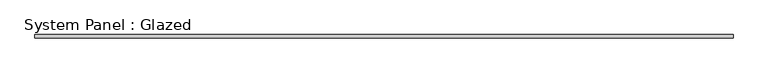
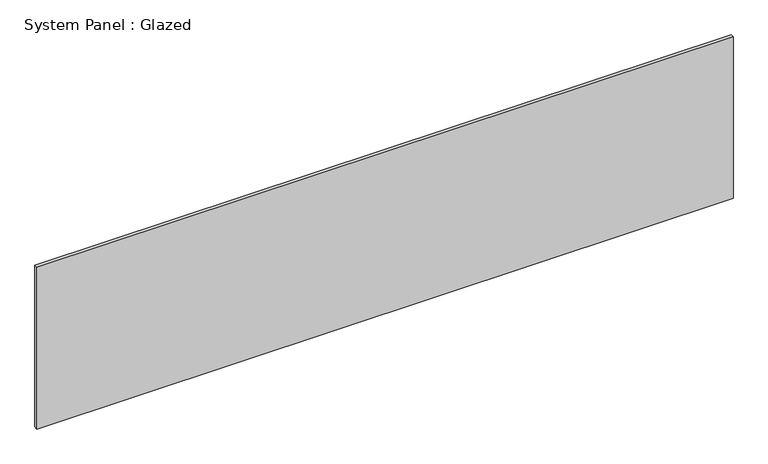
"""IFC4 building model written with IfcOpenShell, lengths in millimetres: plate geometry, System Panel : Glazed."""

from ifc_helpers import new_model, si_unit, origin, origin_with_axes, place, context, project, spatial, polyline, outline, extrude, source, transform, mapped, element, save


def system_panel_glazed_6393fe79(model_context):
    return source(origin(), model_context, "Body", "SweptSolid", [
        extrude(outline(polyline([(2484.742304, 19.05), (-2484.742304, 19.05), (-2484.742304, 44.45), (2484.742304, 44.45), (2484.742304, 19.05)])), origin_with_axes(), (0.0, 0.0, 1.0), 1219.2),
    ])


if __name__ == "__main__":
    model = new_model("IFC4")
    model_context = context("Model", 3, world=origin())
    ifc_project = project(units=[si_unit("LENGTHUNIT", "METRE", prefix="MILLI")], contexts=[model_context])
    site = spatial("IfcSite", under=ifc_project)
    building = spatial("IfcBuilding", under=site)
    placement = place(None, origin())
    system_panel_glazed_shape = system_panel_glazed_6393fe79(model_context)
    element("IfcPlate", 1, ObjectType="System Panel : Glazed", at=placement, inside=building, context=model_context, shape_type="MappedRepresentation", body=[
        mapped(system_panel_glazed_shape, transform((0.0, 0.0, 0.0), x_axis=(1.0, 0.0, 0.0), y_axis=(0.0, 1.0, 0.0), z_axis=(0.0, 0.0, 1.0))),
    ])
    save(model, "model.ifc")

# Revit data of these elements
# Type "System Panel : Glazed"
#   Construction Type Id = "GSP4R"
#   Analytic Construction = "1/8 in Pilkington single glazing"
#   Visual Light Transmittance = 0.9
#   Solar Heat Gain Coefficient = 0.86
#   Heat Transfer Coefficient (U) = 1.18115 BTU/(h·ft²·°F)
# Element 1 (IfcPlate, "System Panel : Glazed")
#   Materials on its faces: "Glass"
# Materials
#   "Glass": class "Glass", colour RGB 0 128 192, transparency 0.75, Description = "Soda Lime Glass", Cost = 0
